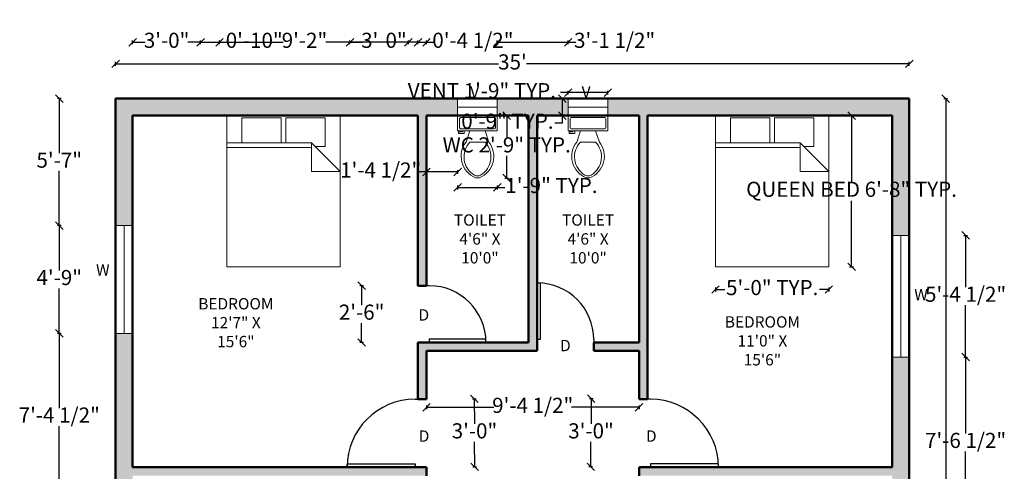
# Model space of a CAD drawing. Units: inches. Extents: x 2395 to 2921, y 528 to 1164.
# Tile 5 of 5: x 2395 to 2916, y 925 to 1164. Entities that reach past the tile are written whole.
import ezdxf

# ---------------------------------------------------------------- set-up
doc = ezdxf.new("R2010")
doc.units = ezdxf.units.IN
for name, color, linetype, lineweight in [('A-ANNO-DIMS', 2, 'Continuous', 18), ('A-ANNO-TEXT', 7, 'Continuous', 18), ('A-AREA-IDEN', 7, 'Continuous', 25), ('A-DOOR', 3, 'Continuous', 25), ('A-FLOR-FIXT', 9, 'Continuous', 18), ('A-FURN', 8, 'Continuous', 18), ('A-GLAZ', 4, 'Continuous', 18), ('A-WALL', 162, 'Continuous', 50), ('A-WALL-PATT', 162, 'Continuous', 13)]:
    doc.layers.add(name, color=color, linetype=linetype, lineweight=lineweight)
doc.styles.get("Standard").update_dxf_attribs({"font": 'arial.ttf'})
doc.dimstyles.new('ISO-25', dxfattribs={"dimtxt": 8, "dimasz": 4, "dimexe": 1, "dimexo": 1, "dimtad": 0, "dimtih": 1, "dimtoh": 1, "dimlunit": 3, "dimtxsty": 'Standard', "dimblk": 'OBLIQUE', "dimcen": 2.5, "dimadec": 0, "dimazin": 0, "dimtfac": 1, "dimtmove": 0, "dimatfit": 3, "dimfxl": 1, "dimfxlon": 1, "dimarcsym": 0})

# ---------------------------------------------------------------- blocks, each defined once
blk = doc.blocks.new('*U6')
for p, q in [((0, 0), (0, -6)), ((30, 0), (30, -6))]:
    blk.add_line(p, q)
blk.add_lwpolyline([(0, 0), (0, 30), (1.75, 30), (1.75, 0)], close=True)
blk.add_arc((0, 0), 30, 0, 90)
blk = doc.blocks.new('*U4')
for p, q in [((-30, 0), (-30, -6)), ((0, 0), (0, -6))]:
    blk.add_line(p, q)
blk.add_lwpolyline([(0, 0), (0, 30), (-1.75, 30), (-1.75, 0)], close=True)
blk.add_arc((0, 0), 30, 90, 180)
blk = doc.blocks.new('*U8')
for p, q in [((0, 0), (0, -6)), ((-36, 0), (-36, -6))]:
    blk.add_line(p, q)
blk.add_lwpolyline([(0, 0), (0, 36), (-1.75, 36), (-1.75, 0)], close=True)
blk.add_arc((0, 0), 36, 90, 180)
blk = doc.blocks.new('*U7')
for p, q in [((0, 0), (0, -6)), ((36, 0), (36, -6))]:
    blk.add_line(p, q)
blk.add_lwpolyline([(0, 0), (0, 36), (1.75, 36), (1.75, 0)], close=True)
blk.add_arc((0, 0), 36, 0, 90)
blk = doc.blocks.new('Toilet - top')
for p, q in [((9.5, -6), (9.5, -2)), ((-10, -8.5), (-8, -8.5)), ((-10, -9.5), (-10, -8.5)), ((-7, -9.5), (-10, -9.5)), ((-8, -8.5), (-8, -8)), ((-7, -8), (-7, -9.5)), ((-4, -8), (-6, -14)), ((4, -8), (6, -14)), ((4, -14), (-4, -14))]:
    blk.add_line(p, q)
blk.add_lwpolyline([(10.5, -8), (10.5, 0), (-10.5, 0), (-10.5, -8)], close=True)
for points in [[(-9.5, -2), (-9.5, -6)], [(8.5, -1), (-8.5, -1)], [(-8.5, -7), (8.5, -7)]]:
    blk.add_lwpolyline(points)
for centre, radius, start, end in [((-8.62, -1.88), 0.884, 81.8699, 188.1301), ((8.62, -1.88), 0.884, 351.8699, 98.1301), ((-8.62, -6.12), 0.884, 171.8699, 278.1301), ((8.62, -6.12), 0.884, 261.8699, 8.1301), ((3.52, -21.58), 12.17, 141.4691, 247.9714), ((4.2, -21.82), 11.33, 136.3677, 238.9468), ((-3.52, -21.58), 12.17, 292.0284, 38.5307), ((-4.2, -21.82), 11.33, 301.053, 43.6321), ((0, -27.88), 4, 245.7318, 294.2682), ((0, -29), 4, 254.8605, 285.1395)]:
    blk.add_arc(centre, radius, start, end)
blk = doc.blocks.new('Bed - Queen')
for p, q in [((0, -80.00003), (0, 0)), ((0, 0), (59.99999, 0)), ((59.99999, 0), (59.99999, -80.00003)), ((7.99999, -1.2), (28.79998, -1.2)), ((7.99999, -14.4), (7.99999, -1.2)), ((28.79998, -1.2), (28.79998, -14.4)), ((31.19999, -1.2), (51.99999, -1.2)), ((31.19999, -14.4), (31.19999, -1.2)), ((51.99999, -1.2), (51.99999, -16.4)), ((0, -14.4), (44.8, -14.4)), ((59.99999, -29.6), (44.8, -14.4)), ((44.8, -14.4), (44.8, -29.6)), ((44.8, -16.8), (0, -16.8)), ((51.99999, -16.4), (46.79936, -16.4)), ((44.8, -29.6), (59.99999, -29.6)), ((59.99999, -80.00003), (0, -80.00003))]:
    blk.add_line(p, q)
blk = doc.blocks.new('_Oblique')
at = {"color": 0, "linetype": 'ByBlock', "lineweight": -2}
blk.add_line((-0.5, -0.5), (0.5, 0.5), dxfattribs=at)
blk = doc.blocks.new('*D19')
at = {"layer": 'A-ANNO-DIMS', "color": 0, "lineweight": -2, "transparency": 16777216}
for p, q in [((2446.2, 1139.21), (2446.2, 1141.21)), ((2866.2, 1139.21), (2866.2, 1141.21)), ((2446.2, 1140.21), (2648.79, 1140.21)), ((2866.2, 1140.21), (2663.61, 1140.21))]:
    blk.add_line(p, q, dxfattribs=at)
at = {"layer": 'Defpoints', "color": 0, "transparency": 16777216}
for p in [(2866.2, 1140.21), (2446.2, 1121.85), (2866.2, 1121.85)]:
    blk.add_point(p, dxfattribs=at)
at = {"layer": 'A-ANNO-DIMS', "color": 0, "lineweight": -2, "transparency": 16777216, "xscale": 4, "yscale": 4, "zscale": 4, "rotation": 180}
blk.add_blockref('_Oblique', (2446.2, 1140.21), dxfattribs=at)
at = {"layer": 'A-ANNO-DIMS', "color": 0, "lineweight": -2, "transparency": 16777216, "xscale": 4, "yscale": 4, "zscale": 4}
blk.add_blockref('_Oblique', (2866.2, 1140.21), dxfattribs=at)
at = {"layer": 'A-ANNO-DIMS', "color": 0, "transparency": 16777216, "insert": (2656.2, 1140.21), "char_height": 8, "attachment_point": 5}
blk.add_mtext("35'", dxfattribs=at)
blk = doc.blocks.new('*D20')
at = {"layer": 'A-ANNO-DIMS', "color": 0, "lineweight": -2, "transparency": 16777216}
for p, q in [((2884.49, 1121.85), (2886.49, 1121.85)), ((2885.49, 1121.85), (2885.49, 850.56)), ((2885.49, 569.85), (2885.49, 841.14)), ((2884.49, 569.85), (2886.49, 569.85))]:
    blk.add_line(p, q, dxfattribs=at)
at = {"layer": 'Defpoints', "color": 0, "transparency": 16777216}
for p in [(2866.2, 1121.85), (2866.2, 569.85), (2885.49, 569.85)]:
    blk.add_point(p, dxfattribs=at)
at = {"layer": 'A-ANNO-DIMS', "color": 0, "lineweight": -2, "transparency": 16777216, "xscale": 4, "yscale": 4, "zscale": 4}
for p, rotation in [((2885.49, 1121.85), 90), ((2885.49, 569.85), 270)]:
    blk.add_blockref('_Oblique', p, dxfattribs=dict(at, rotation=rotation))
at = {"layer": 'A-ANNO-DIMS', "color": 0, "transparency": 16777216, "insert": (2885.49, 845.85), "char_height": 8, "attachment_point": 5}
blk.add_mtext("46'", dxfattribs=at)
blk = doc.blocks.new('VENT-WINDOW-21IN')
for p, q in [((0, 0), (0, 9)), ((21, 0), (21, 9)), ((0, 4.5), (21, 4.5))]:
    blk.add_line(p, q)
blk = doc.blocks.new('*D22')
at = {"layer": 'A-ANNO-DIMS', "color": 0, "lineweight": -2, "transparency": 16777216}
for p, q in [((2834.65, 1112.85), (2836.65, 1112.85)), ((2835.65, 1112.85), (2835.65, 1077.86)), ((2835.65, 1032.85), (2835.65, 1067.85)), ((2834.65, 1032.85), (2836.65, 1032.85))]:
    blk.add_line(p, q, dxfattribs=at)
at = {"layer": 'Defpoints', "color": 0, "transparency": 16777216}
for p in [(2823.65, 1112.85), (2835.65, 1112.85), (2823.65, 1032.85)]:
    blk.add_point(p, dxfattribs=at)
at = {"layer": 'A-ANNO-DIMS', "color": 0, "lineweight": -2, "transparency": 16777216, "xscale": 4, "yscale": 4, "zscale": 4}
for p, rotation in [((2835.65, 1112.85), 90), ((2835.65, 1032.85), 270)]:
    blk.add_blockref('_Oblique', p, dxfattribs=dict(at, rotation=rotation))
at = {"layer": 'A-ANNO-DIMS', "color": 0, "transparency": 16777216, "insert": (2835.65, 1072.85), "char_height": 8, "attachment_point": 5}
blk.add_mtext('QUEEN BED 6\'-8" TYP.', dxfattribs=at)
blk = doc.blocks.new('*D23')
at = {"layer": 'A-ANNO-DIMS', "color": 0, "lineweight": -2, "transparency": 16777216}
for p, q in [((2763.65, 1021.85), (2763.65, 1019.85)), ((2823.65, 1021.85), (2823.65, 1019.85)), ((2763.65, 1020.85), (2768.64, 1020.85)), ((2823.65, 1020.85), (2818.66, 1020.85))]:
    blk.add_line(p, q, dxfattribs=at)
at = {"layer": 'Defpoints', "color": 0, "transparency": 16777216}
for p in [(2763.65, 1032.85), (2823.65, 1032.85), (2823.65, 1020.85)]:
    blk.add_point(p, dxfattribs=at)
at = {"layer": 'A-ANNO-DIMS', "color": 0, "lineweight": -2, "transparency": 16777216, "xscale": 4, "yscale": 4, "zscale": 4, "rotation": 180}
blk.add_blockref('_Oblique', (2763.65, 1020.85), dxfattribs=at)
at = {"layer": 'A-ANNO-DIMS', "color": 0, "lineweight": -2, "transparency": 16777216, "xscale": 4, "yscale": 4, "zscale": 4}
blk.add_blockref('_Oblique', (2823.65, 1020.85), dxfattribs=at)
at = {"layer": 'A-ANNO-DIMS', "color": 0, "transparency": 16777216, "insert": (2793.65, 1020.85), "char_height": 8, "attachment_point": 5}
blk.add_mtext('5\'-0" TYP.', dxfattribs=at)
blk = doc.blocks.new('*D24')
at = {"layer": 'A-ANNO-DIMS', "color": 0, "lineweight": -2, "transparency": 16777216}
for p, q in [((2652.16, 1112.85), (2654.16, 1112.85)), ((2653.16, 1112.85), (2653.16, 1101.09)), ((2653.16, 1079.81), (2653.16, 1091.57)), ((2652.16, 1079.81), (2654.16, 1079.81))]:
    blk.add_line(p, q, dxfattribs=at)
at = {"layer": 'Defpoints', "color": 0, "transparency": 16777216}
for p in [(2648.2, 1112.85), (2653.16, 1112.85), (2648.2, 1079.81)]:
    blk.add_point(p, dxfattribs=at)
at = {"layer": 'A-ANNO-DIMS', "color": 0, "lineweight": -2, "transparency": 16777216, "xscale": 4, "yscale": 4, "zscale": 4}
for p, rotation in [((2653.16, 1112.85), 90), ((2653.16, 1079.81), 270)]:
    blk.add_blockref('_Oblique', p, dxfattribs=dict(at, rotation=rotation))
at = {"layer": 'A-ANNO-DIMS', "color": 0, "transparency": 16777216, "insert": (2653.16, 1096.33), "char_height": 8, "attachment_point": 5}
blk.add_mtext('WC 2\'-9" TYP.', dxfattribs=at)
blk = doc.blocks.new('*D25')
at = {"layer": 'A-ANNO-DIMS', "color": 0, "lineweight": -2, "transparency": 16777216}
for p, q in [((2627.2, 1075.85), (2627.2, 1073.85)), ((2627.2, 1074.85), (2648.2, 1074.85)), ((2648.2, 1075.85), (2648.2, 1073.85)), ((2648.2, 1074.85), (2652.2, 1074.85))]:
    blk.add_line(p, q, dxfattribs=at)
at = {"layer": 'Defpoints', "color": 0, "transparency": 16777216}
for p in [(2627.2, 1079.81), (2648.2, 1079.81), (2648.2, 1074.85)]:
    blk.add_point(p, dxfattribs=at)
at = {"layer": 'A-ANNO-DIMS', "color": 0, "lineweight": -2, "transparency": 16777216, "xscale": 4, "yscale": 4, "zscale": 4, "rotation": 180}
blk.add_blockref('_Oblique', (2627.2, 1074.85), dxfattribs=at)
at = {"layer": 'A-ANNO-DIMS', "color": 0, "lineweight": -2, "transparency": 16777216, "xscale": 4, "yscale": 4, "zscale": 4}
blk.add_blockref('_Oblique', (2648.2, 1074.85), dxfattribs=at)
at = {"layer": 'A-ANNO-DIMS', "color": 0, "transparency": 16777216, "insert": (2676.83, 1074.85), "char_height": 8, "attachment_point": 5}
blk.add_mtext('1\'-9" TYP.', dxfattribs=at)
blk = doc.blocks.new('*D26')
at = {"layer": 'A-ANNO-DIMS', "color": 0, "lineweight": -2, "transparency": 16777216}
for p, q in [((2685.7, 1124), (2685.7, 1126)), ((2706.7, 1124), (2706.7, 1126)), ((2685.7, 1125), (2681.7, 1125)), ((2706.7, 1125), (2685.7, 1125))]:
    blk.add_line(p, q, dxfattribs=at)
at = {"layer": 'Defpoints', "color": 0, "transparency": 16777216}
for p in [(2685.7, 1125), (2685.7, 1121.85), (2706.7, 1121.85)]:
    blk.add_point(p, dxfattribs=at)
at = {"layer": 'A-ANNO-DIMS', "color": 0, "lineweight": -2, "transparency": 16777216, "xscale": 4, "yscale": 4, "zscale": 4, "rotation": 180}
blk.add_blockref('_Oblique', (2685.7, 1125), dxfattribs=at)
at = {"layer": 'A-ANNO-DIMS', "color": 0, "lineweight": -2, "transparency": 16777216, "xscale": 4, "yscale": 4, "zscale": 4}
blk.add_blockref('_Oblique', (2706.7, 1125), dxfattribs=at)
at = {"layer": 'A-ANNO-DIMS', "color": 0, "transparency": 16777216, "insert": (2640.03, 1125), "char_height": 8, "attachment_point": 5}
blk.add_mtext('VENT 1\'-9" TYP.', dxfattribs=at)
blk = doc.blocks.new('*D27')
at = {"layer": 'A-ANNO-DIMS', "color": 0, "lineweight": -2, "transparency": 16777216}
for p, q in [((2683.55, 1121.85), (2681.55, 1121.85)), ((2682.55, 1121.85), (2682.55, 1112.85)), ((2683.55, 1112.85), (2681.55, 1112.85)), ((2682.55, 1112.85), (2682.55, 1108.85)), ((2682.55, 1108.85), (2678.55, 1108.85))]:
    blk.add_line(p, q, dxfattribs=at)
at = {"layer": 'Defpoints', "color": 0, "transparency": 16777216}
for p in [(2685.7, 1121.85), (2682.55, 1112.85), (2685.7, 1112.85)]:
    blk.add_point(p, dxfattribs=at)
at = {"layer": 'A-ANNO-DIMS', "color": 0, "lineweight": -2, "transparency": 16777216, "xscale": 4, "yscale": 4, "zscale": 4}
for p, rotation in [((2682.55, 1121.85), 90), ((2682.55, 1112.85), 270)]:
    blk.add_blockref('_Oblique', p, dxfattribs=dict(at, rotation=rotation))
at = {"layer": 'A-ANNO-DIMS', "color": 0, "transparency": 16777216, "insert": (2653.54, 1108.85), "char_height": 8, "attachment_point": 5}
blk.add_mtext('0\'-9" TYP.', dxfattribs=at)
blk = doc.blocks.new('*D51')
at = {"layer": 'A-ANNO-DIMS', "color": 0, "lineweight": -2, "transparency": 16777216}
for p, q in [((2606.2, 1150.65), (2606.2, 1152.65)), ((2606.2, 1151.65), (2610.7, 1151.65)), ((2610.7, 1150.65), (2610.7, 1152.65)), ((2610.7, 1151.65), (2614.7, 1151.65))]:
    blk.add_line(p, q, dxfattribs=at)
at = {"layer": 'Defpoints', "color": 0, "transparency": 16777216}
for p in [(2610.7, 1151.65), (2606.2, 578.85), (2610.7, 578.85)]:
    blk.add_point(p, dxfattribs=at)
at = {"layer": 'A-ANNO-DIMS', "color": 0, "lineweight": -2, "transparency": 16777216, "xscale": 4, "yscale": 4, "zscale": 4, "rotation": 180}
blk.add_blockref('_Oblique', (2606.2, 1151.65), dxfattribs=at)
at = {"layer": 'A-ANNO-DIMS', "color": 0, "lineweight": -2, "transparency": 16777216, "xscale": 4, "yscale": 4, "zscale": 4}
blk.add_blockref('_Oblique', (2610.7, 1151.65), dxfattribs=at)
at = {"layer": 'A-ANNO-DIMS', "color": 0, "transparency": 16777216, "insert": (2635.28, 1151.65), "char_height": 8, "attachment_point": 5}
blk.add_mtext('0\'-4 1/2"', dxfattribs=at)
blk = doc.blocks.new('*D53')
at = {"layer": 'A-ANNO-DIMS', "color": 0, "lineweight": -2, "transparency": 16777216}
for p, q in [((2455.2, 1150.65), (2455.2, 1152.65)), ((2455.2, 1151.65), (2461.94, 1151.65)), ((2491.2, 1151.65), (2484.46, 1151.65)), ((2491.2, 1150.65), (2491.2, 1152.65))]:
    blk.add_line(p, q, dxfattribs=at)
at = {"layer": 'Defpoints', "color": 0, "transparency": 16777216}
for p in [(2491.2, 1151.65), (2455.2, 922.35), (2491.2, 922.35)]:
    blk.add_point(p, dxfattribs=at)
at = {"layer": 'A-ANNO-DIMS', "color": 0, "lineweight": -2, "transparency": 16777216, "xscale": 4, "yscale": 4, "zscale": 4, "rotation": 180}
blk.add_blockref('_Oblique', (2455.2, 1151.65), dxfattribs=at)
at = {"layer": 'A-ANNO-DIMS', "color": 0, "lineweight": -2, "transparency": 16777216, "xscale": 4, "yscale": 4, "zscale": 4}
blk.add_blockref('_Oblique', (2491.2, 1151.65), dxfattribs=at)
at = {"layer": 'A-ANNO-DIMS', "color": 0, "transparency": 16777216, "insert": (2473.2, 1151.65), "char_height": 8, "attachment_point": 5}
blk.add_mtext('3\'-0"', dxfattribs=at)
blk = doc.blocks.new('*D54')
at = {"layer": 'A-ANNO-DIMS', "color": 0, "lineweight": -2, "transparency": 16777216}
for p, q in [((2491.2, 1150.65), (2491.2, 1152.65)), ((2491.2, 1151.65), (2534.91, 1151.65)), ((2601.13, 1151.65), (2557.42, 1151.65)), ((2601.13, 1150.65), (2601.13, 1152.65))]:
    blk.add_line(p, q, dxfattribs=at)
at = {"layer": 'Defpoints', "color": 0, "transparency": 16777216}
for p in [(2601.13, 1151.65), (2491.2, 922.35), (2601.13, 922.35)]:
    blk.add_point(p, dxfattribs=at)
at = {"layer": 'A-ANNO-DIMS', "color": 0, "lineweight": -2, "transparency": 16777216, "xscale": 4, "yscale": 4, "zscale": 4, "rotation": 180}
blk.add_blockref('_Oblique', (2491.2, 1151.65), dxfattribs=at)
at = {"layer": 'A-ANNO-DIMS', "color": 0, "lineweight": -2, "transparency": 16777216, "xscale": 4, "yscale": 4, "zscale": 4}
blk.add_blockref('_Oblique', (2601.13, 1151.65), dxfattribs=at)
at = {"layer": 'A-ANNO-DIMS', "color": 0, "transparency": 16777216, "insert": (2546.16, 1151.65), "char_height": 8, "attachment_point": 5}
blk.add_mtext('9\'-2"', dxfattribs=at)
blk = doc.blocks.new('*D55')
at = {"layer": 'A-ANNO-DIMS', "color": 0, "lineweight": -2, "transparency": 16777216}
for p, q in [((2491.2, 1150.65), (2491.2, 1152.65)), ((2491.2, 1151.65), (2501.19, 1151.65)), ((2501.19, 1150.65), (2501.19, 1152.65)), ((2501.19, 1151.65), (2505.19, 1151.65))]:
    blk.add_line(p, q, dxfattribs=at)
at = {"layer": 'Defpoints', "color": 0, "transparency": 16777216}
for p in [(2501.19, 1151.65), (2491.2, 842.85), (2501.19, 842.85)]:
    blk.add_point(p, dxfattribs=at)
at = {"layer": 'A-ANNO-DIMS', "color": 0, "lineweight": -2, "transparency": 16777216, "xscale": 4, "yscale": 4, "zscale": 4, "rotation": 180}
blk.add_blockref('_Oblique', (2491.2, 1151.65), dxfattribs=at)
at = {"layer": 'A-ANNO-DIMS', "color": 0, "lineweight": -2, "transparency": 16777216, "xscale": 4, "yscale": 4, "zscale": 4}
blk.add_blockref('_Oblique', (2501.19, 1151.65), dxfattribs=at)
at = {"layer": 'A-ANNO-DIMS', "color": 0, "transparency": 16777216, "insert": (2519.56, 1151.65), "char_height": 8, "attachment_point": 5}
blk.add_mtext('0\'-10"', dxfattribs=at)
blk = doc.blocks.new('*D56')
at = {"layer": 'A-ANNO-DIMS', "color": 0, "lineweight": -2, "transparency": 16777216}
for p, q in [((2417.4, 1121.85), (2415.4, 1121.85)), ((2416.4, 1121.85), (2416.4, 1092.94)), ((2416.4, 1054.65), (2416.4, 1083.56)), ((2417.4, 1054.65), (2415.4, 1054.65))]:
    blk.add_line(p, q, dxfattribs=at)
at = {"layer": 'Defpoints', "color": 0, "transparency": 16777216}
for p in [(2446.2, 1121.85), (2416.4, 1054.65), (2446.2, 1054.65)]:
    blk.add_point(p, dxfattribs=at)
at = {"layer": 'A-ANNO-DIMS', "color": 0, "lineweight": -2, "transparency": 16777216, "xscale": 4, "yscale": 4, "zscale": 4}
for p, rotation in [((2416.4, 1121.85), 90), ((2416.4, 1054.65), 270)]:
    blk.add_blockref('_Oblique', p, dxfattribs=dict(at, rotation=rotation))
at = {"layer": 'A-ANNO-DIMS', "color": 0, "transparency": 16777216, "insert": (2416.4, 1088.25), "char_height": 8, "attachment_point": 5}
blk.add_mtext('5\'-7"', dxfattribs=at)
blk = doc.blocks.new('*D57')
at = {"layer": 'A-ANNO-DIMS', "color": 0, "lineweight": -2, "transparency": 16777216}
for p, q in [((2417.4, 1054.65), (2415.4, 1054.65)), ((2416.4, 1054.65), (2416.4, 1030.86)), ((2416.4, 997.65), (2416.4, 1021.44)), ((2417.4, 997.65), (2415.4, 997.65))]:
    blk.add_line(p, q, dxfattribs=at)
at = {"layer": 'Defpoints', "color": 0, "transparency": 16777216}
for p in [(2446.2, 1054.65), (2416.4, 997.65), (2446.2, 997.65)]:
    blk.add_point(p, dxfattribs=at)
at = {"layer": 'A-ANNO-DIMS', "color": 0, "lineweight": -2, "transparency": 16777216, "xscale": 4, "yscale": 4, "zscale": 4}
for p, rotation in [((2416.4, 1054.65), 90), ((2416.4, 997.65), 270)]:
    blk.add_blockref('_Oblique', p, dxfattribs=dict(at, rotation=rotation))
at = {"layer": 'A-ANNO-DIMS', "color": 0, "transparency": 16777216, "insert": (2416.4, 1026.15), "char_height": 8, "attachment_point": 5}
blk.add_mtext('4\'-9"', dxfattribs=at)
blk = doc.blocks.new('*D58')
at = {"layer": 'A-ANNO-DIMS', "color": 0, "lineweight": -2, "transparency": 16777216}
for p, q in [((2417.4, 997.65), (2415.4, 997.65)), ((2416.4, 997.65), (2416.4, 958.18)), ((2416.4, 909.18), (2416.4, 948.66)), ((2417.4, 909.18), (2415.4, 909.18))]:
    blk.add_line(p, q, dxfattribs=at)
at = {"layer": 'Defpoints', "color": 0, "transparency": 16777216}
for p in [(2446.2, 997.65), (2416.4, 909.18), (2446.2, 909.18)]:
    blk.add_point(p, dxfattribs=at)
at = {"layer": 'A-ANNO-DIMS', "color": 0, "lineweight": -2, "transparency": 16777216, "xscale": 4, "yscale": 4, "zscale": 4}
for p, rotation in [((2416.4, 997.65), 90), ((2416.4, 909.18), 270)]:
    blk.add_blockref('_Oblique', p, dxfattribs=dict(at, rotation=rotation))
at = {"layer": 'A-ANNO-DIMS', "color": 0, "transparency": 16777216, "insert": (2416.4, 953.42), "char_height": 8, "attachment_point": 5}
blk.add_mtext('7\'-4 1/2"', dxfattribs=at)
blk = doc.blocks.new('*D68')
at = {"layer": 'A-ANNO-DIMS', "color": 0, "lineweight": -2, "transparency": 16777216}
for p, q in [((2895, 985.13), (2897, 985.13)), ((2896, 985.13), (2896, 944.76)), ((2896, 894.87), (2896, 935.24)), ((2895, 894.87), (2897, 894.87))]:
    blk.add_line(p, q, dxfattribs=at)
at = {"layer": 'Defpoints', "color": 0, "transparency": 16777216}
for p in [(2866.2, 985.13), (2896, 985.13), (2866.2, 894.87)]:
    blk.add_point(p, dxfattribs=at)
at = {"layer": 'A-ANNO-DIMS', "color": 0, "lineweight": -2, "transparency": 16777216, "xscale": 4, "yscale": 4, "zscale": 4}
for p, rotation in [((2896, 985.13), 90), ((2896, 894.87), 270)]:
    blk.add_blockref('_Oblique', p, dxfattribs=dict(at, rotation=rotation))
at = {"layer": 'A-ANNO-DIMS', "color": 0, "transparency": 16777216, "insert": (2896, 940), "char_height": 8, "attachment_point": 5}
blk.add_mtext('7\'-6 1/2"', dxfattribs=at)
blk = doc.blocks.new('*D69')
at = {"layer": 'A-ANNO-DIMS', "color": 0, "lineweight": -2, "transparency": 16777216}
for p, q in [((2895, 1049.51), (2897, 1049.51)), ((2896, 1049.51), (2896, 1022.08)), ((2896, 985.13), (2896, 1012.56)), ((2895, 985.13), (2897, 985.13))]:
    blk.add_line(p, q, dxfattribs=at)
at = {"layer": 'Defpoints', "color": 0, "transparency": 16777216}
for p in [(2866.2, 1049.51), (2896, 1049.51), (2866.2, 985.13)]:
    blk.add_point(p, dxfattribs=at)
at = {"layer": 'A-ANNO-DIMS', "color": 0, "lineweight": -2, "transparency": 16777216, "xscale": 4, "yscale": 4, "zscale": 4}
for p, rotation in [((2896, 1049.51), 90), ((2896, 985.13), 270)]:
    blk.add_blockref('_Oblique', p, dxfattribs=dict(at, rotation=rotation))
at = {"layer": 'A-ANNO-DIMS', "color": 0, "transparency": 16777216, "insert": (2896, 1017.32), "char_height": 8, "attachment_point": 5}
blk.add_mtext('5\'-4 1/2"', dxfattribs=at)
blk = doc.blocks.new('*D70')
at = {"layer": 'A-ANNO-DIMS', "color": 0, "lineweight": -2, "transparency": 16777216}
for p, q in [((2610.7, 1084.05), (2610.7, 1082.05)), ((2627.2, 1084.05), (2627.2, 1082.05)), ((2610.7, 1083.05), (2606.7, 1083.05)), ((2627.2, 1083.05), (2610.7, 1083.05))]:
    blk.add_line(p, q, dxfattribs=at)
at = {"layer": 'Defpoints', "color": 0, "transparency": 16777216}
for p in [(2610.7, 1112.85), (2627.2, 1112.85), (2610.7, 1083.05)]:
    blk.add_point(p, dxfattribs=at)
at = {"layer": 'A-ANNO-DIMS', "color": 0, "lineweight": -2, "transparency": 16777216, "xscale": 4, "yscale": 4, "zscale": 4, "rotation": 180}
blk.add_blockref('_Oblique', (2610.7, 1083.05), dxfattribs=at)
at = {"layer": 'A-ANNO-DIMS', "color": 0, "lineweight": -2, "transparency": 16777216, "xscale": 4, "yscale": 4, "zscale": 4}
blk.add_blockref('_Oblique', (2627.2, 1083.05), dxfattribs=at)
at = {"layer": 'A-ANNO-DIMS', "color": 0, "transparency": 16777216, "insert": (2586.5, 1083.05), "char_height": 8, "attachment_point": 5}
blk.add_mtext('1\'-4 1/2"', dxfattribs=at)
blk = doc.blocks.new('*D71')
at = {"layer": 'A-ANNO-DIMS', "color": 0, "lineweight": -2, "transparency": 16777216}
for p, q in [((2648.2, 1150.65), (2648.2, 1152.65)), ((2648.2, 1151.65), (2685.7, 1151.65)), ((2685.7, 1150.65), (2685.7, 1152.65)), ((2685.7, 1151.65), (2689.7, 1151.65))]:
    blk.add_line(p, q, dxfattribs=at)
at = {"layer": 'Defpoints', "color": 0, "transparency": 16777216}
for p in [(2685.7, 1151.65), (2648.2, 1121.85), (2685.7, 1121.85)]:
    blk.add_point(p, dxfattribs=at)
at = {"layer": 'A-ANNO-DIMS', "color": 0, "lineweight": -2, "transparency": 16777216, "xscale": 4, "yscale": 4, "zscale": 4, "rotation": 180}
blk.add_blockref('_Oblique', (2648.2, 1151.65), dxfattribs=at)
at = {"layer": 'A-ANNO-DIMS', "color": 0, "lineweight": -2, "transparency": 16777216, "xscale": 4, "yscale": 4, "zscale": 4}
blk.add_blockref('_Oblique', (2685.7, 1151.65), dxfattribs=at)
at = {"layer": 'A-ANNO-DIMS', "color": 0, "transparency": 16777216, "insert": (2710.28, 1151.65), "char_height": 8, "attachment_point": 5}
blk.add_mtext('3\'-1 1/2"', dxfattribs=at)
blk = doc.blocks.new('*D72')
at = {"layer": 'A-ANNO-DIMS', "color": 0, "lineweight": -2, "transparency": 16777216}
for p, q in [((2577.4, 1022.85), (2575.4, 1022.85)), ((2576.4, 1022.85), (2576.4, 1012.56)), ((2576.4, 992.85), (2576.4, 1003.14)), ((2577.4, 992.85), (2575.4, 992.85))]:
    blk.add_line(p, q, dxfattribs=at)
at = {"layer": 'Defpoints', "color": 0, "transparency": 16777216}
for p in [(2576.4, 1022.85), (2606.2, 1022.85), (2606.2, 992.85)]:
    blk.add_point(p, dxfattribs=at)
at = {"layer": 'A-ANNO-DIMS', "color": 0, "lineweight": -2, "transparency": 16777216, "xscale": 4, "yscale": 4, "zscale": 4}
for p, rotation in [((2576.4, 1022.85), 90), ((2576.4, 992.85), 270)]:
    blk.add_blockref('_Oblique', p, dxfattribs=dict(at, rotation=rotation))
at = {"layer": 'A-ANNO-DIMS', "color": 0, "transparency": 16777216, "insert": (2576.4, 1007.85), "char_height": 8, "attachment_point": 5}
blk.add_mtext('2\'-6"', dxfattribs=at)
blk = doc.blocks.new('*D73')
at = {"layer": 'A-ANNO-DIMS', "color": 0, "lineweight": -2, "transparency": 16777216}
for p, q in [((2669.2, 541.05), (2669.2, 539.05)), ((2669.2, 540.05), (2672.87, 540.05)), ((2699.2, 540.05), (2695.53, 540.05)), ((2699.2, 541.05), (2699.2, 539.05))]:
    blk.add_line(p, q, dxfattribs=at)
at = {"layer": 'Defpoints', "color": 0, "transparency": 16777216}
for p in [(2669.2, 988.35), (2699.2, 988.35), (2699.2, 540.05)]:
    blk.add_point(p, dxfattribs=at)
at = {"layer": 'A-ANNO-DIMS', "color": 0, "lineweight": -2, "transparency": 16777216, "xscale": 4, "yscale": 4, "zscale": 4, "rotation": 180}
blk.add_blockref('_Oblique', (2669.2, 540.05), dxfattribs=at)
at = {"layer": 'A-ANNO-DIMS', "color": 0, "lineweight": -2, "transparency": 16777216, "xscale": 4, "yscale": 4, "zscale": 4}
blk.add_blockref('_Oblique', (2699.2, 540.05), dxfattribs=at)
at = {"layer": 'A-ANNO-DIMS', "color": 0, "transparency": 16777216, "insert": (2684.2, 540.05), "char_height": 8, "attachment_point": 5}
blk.add_mtext('2\'-6"', dxfattribs=at)
blk = doc.blocks.new('*D74')
at = {"layer": 'A-ANNO-DIMS', "color": 0, "lineweight": -2, "transparency": 16777216}
for p, q in [((2635, 963.05), (2637, 963.07)), ((2636, 963.06), (2636.09, 949.77)), ((2636.25, 927.06), (2636.16, 940.35)), ((2635.25, 927.05), (2637.25, 927.07))]:
    blk.add_line(p, q, dxfattribs=at)
at = {"layer": 'Defpoints', "color": 0, "transparency": 16777216}
for p in [(2606.2, 962.85), (2606.45, 926.85), (2636.25, 927.06)]:
    blk.add_point(p, dxfattribs=at)
at = {"layer": 'A-ANNO-DIMS', "color": 0, "lineweight": -2, "transparency": 16777216, "xscale": 4, "yscale": 4, "zscale": 4}
for p, rotation in [((2636, 963.06), 90.39788096183455), ((2636.25, 927.06), 270.3978809618346)]:
    blk.add_blockref('_Oblique', p, dxfattribs=dict(at, rotation=rotation))
at = {"layer": 'A-ANNO-DIMS', "color": 0, "transparency": 16777216, "insert": (2636.12, 945.06), "char_height": 8, "attachment_point": 5}
blk.add_mtext('3\'-0"', dxfattribs=at)
blk = doc.blocks.new('*D75')
at = {"layer": 'A-ANNO-DIMS', "color": 0, "lineweight": -2, "transparency": 16777216}
for p, q in [((2698.9, 963.05), (2696.9, 963.07)), ((2697.9, 963.06), (2697.81, 949.77)), ((2697.65, 927.06), (2697.74, 940.35)), ((2698.65, 927.05), (2696.65, 927.07))]:
    blk.add_line(p, q, dxfattribs=at)
at = {"layer": 'Defpoints', "color": 0, "transparency": 16777216}
for p in [(2697.9, 963.06), (2727.7, 962.85), (2727.45, 926.85)]:
    blk.add_point(p, dxfattribs=at)
at = {"layer": 'A-ANNO-DIMS', "color": 0, "lineweight": -2, "transparency": 16777216, "xscale": 4, "yscale": 4, "zscale": 4}
for p, rotation in [((2697.9, 963.06), 89.6021190381654), ((2697.65, 927.06), 269.6021190381654)]:
    blk.add_blockref('_Oblique', p, dxfattribs=dict(at, rotation=rotation))
at = {"layer": 'A-ANNO-DIMS', "color": 0, "transparency": 16777216, "insert": (2697.78, 945.06), "char_height": 8, "attachment_point": 5}
blk.add_mtext('3\'-0"', dxfattribs=at)
blk = doc.blocks.new('*D78')
at = {"layer": 'A-ANNO-DIMS', "color": 0, "lineweight": -2, "transparency": 16777216}
for p, q in [((2570.2, 1150.65), (2570.2, 1152.65)), ((2570.2, 1151.65), (2576.94, 1151.65)), ((2606.2, 1151.65), (2599.46, 1151.65)), ((2606.2, 1150.65), (2606.2, 1152.65))]:
    blk.add_line(p, q, dxfattribs=at)
at = {"layer": 'Defpoints', "color": 0, "transparency": 16777216}
for p in [(2606.2, 1151.65), (2570.2, 734.85), (2606.2, 735.1)]:
    blk.add_point(p, dxfattribs=at)
at = {"layer": 'A-ANNO-DIMS', "color": 0, "lineweight": -2, "transparency": 16777216, "xscale": 4, "yscale": 4, "zscale": 4, "rotation": 180}
blk.add_blockref('_Oblique', (2570.2, 1151.65), dxfattribs=at)
at = {"layer": 'A-ANNO-DIMS', "color": 0, "lineweight": -2, "transparency": 16777216, "xscale": 4, "yscale": 4, "zscale": 4}
blk.add_blockref('_Oblique', (2606.2, 1151.65), dxfattribs=at)
at = {"layer": 'A-ANNO-DIMS', "color": 0, "transparency": 16777216, "insert": (2588.2, 1151.65), "char_height": 8, "attachment_point": 5}
blk.add_mtext('3\'-0"', dxfattribs=at)
blk = doc.blocks.new('*D79')
at = {"layer": 'A-ANNO-DIMS', "color": 0, "lineweight": -2, "transparency": 16777216}
for p, q in [((2610.7, 959.55), (2610.7, 957.55)), ((2723.2, 959.55), (2723.2, 957.55)), ((2610.7, 958.55), (2646.37, 958.55)), ((2723.2, 958.55), (2687.53, 958.55))]:
    blk.add_line(p, q, dxfattribs=at)
at = {"layer": 'Defpoints', "color": 0, "transparency": 16777216}
for p in [(2610.7, 988.35), (2723.2, 988.35), (2610.7, 958.55)]:
    blk.add_point(p, dxfattribs=at)
at = {"layer": 'A-ANNO-DIMS', "color": 0, "lineweight": -2, "transparency": 16777216, "xscale": 4, "yscale": 4, "zscale": 4, "rotation": 180}
blk.add_blockref('_Oblique', (2610.7, 958.55), dxfattribs=at)
at = {"layer": 'A-ANNO-DIMS', "color": 0, "lineweight": -2, "transparency": 16777216, "xscale": 4, "yscale": 4, "zscale": 4}
blk.add_blockref('_Oblique', (2723.2, 958.55), dxfattribs=at)
at = {"layer": 'A-ANNO-DIMS', "color": 0, "transparency": 16777216, "insert": (2666.95, 958.55), "char_height": 8, "attachment_point": 5}
blk.add_mtext('9\'-4 1/2"', dxfattribs=at)

msp = doc.modelspace()

# ---------------------------------------------------------------- hatches: boundary and pattern name
at = {"layer": 'A-WALL-PATT'}
h = msp.add_hatch(color=256, dxfattribs=at)
h.dxf.hatch_style = 1
h.paths.add_polyline_path([(2627.2, 1121.853), (2446.2, 1121.853), (2446.2, 1054.648), (2455.2, 1054.648), (2455.2, 1112.853), (2606.2, 1112.853), (2606.2, 1022.853), (2610.7, 1022.853), (2610.7, 1112.853), (2627.2, 1112.853)])
h.paths.add_polyline_path([(2685.7, 1121.853), (2648.2, 1121.853), (2648.2, 1112.853), (2664.7, 1112.853), (2664.7, 992.853), (2606.2, 992.853), (2606.2, 962.853), (2610.7, 962.853), (2610.7, 988.353), (2669.2, 988.353), (2669.2, 994.353), (2669.2, 1024.353), (2669.2, 1112.853), (2685.7, 1112.853)])
h.paths.add_polyline_path([(2866.2, 1121.853), (2706.7, 1121.853), (2706.7, 1112.853), (2723.2, 1112.853), (2723.2, 992.853), (2699.2, 992.853), (2699.2, 988.353), (2723.2, 988.353), (2723.2, 962.853), (2727.7, 962.853), (2727.7, 1112.853), (2857.2, 1112.853), (2857.2, 1049.508), (2866.2, 1049.508)])
h.paths.add_polyline_path([(2866.2, 985.129), (2857.2, 985.129), (2857.2, 926.853), (2723.2, 926.853), (2723.2, 922.353), (2729.2, 922.353), (2765.2, 922.353), (2857.2, 922.353), (2857.2, 894.873), (2866.2, 894.873)])
h.paths.add_polyline_path([(2455.2, 997.652), (2446.2, 997.652), (2446.2, 909.181), (2455.2, 908.938), (2455.2, 922.353), (2610.7, 922.353), (2610.7, 926.853), (2455.2, 926.853)])
h.paths.add_polyline_path([(2455.2, 838.353), (2610.7, 838.353), (2610.7, 842.853), (2455.2, 842.853), (2455.2, 856.236), (2446.2, 856.236), (2446.2, 815.427), (2455.2, 815.427)])
h.paths.add_polyline_path([(2455.2, 772.706), (2446.2, 772.706), (2446.2, 569.853), (2505.031, 569.853), (2505.031, 578.853), (2455.2, 578.853), (2455.2, 734.853), (2570.2, 734.853), (2570.2, 739.353), (2568.7, 739.353), (2568.7, 806.353), (2564.2, 806.353), (2564.2, 739.353), (2455.2, 739.353)])
h.paths.add_polyline_path([(2656.2, 578.853), (2610.7, 578.853), (2610.7, 739.353), (2606.2, 739.353), (2606.2, 578.853), (2565.031, 578.853), (2565.031, 569.853), (2656.2, 569.853)])
h.paths.add_polyline_path([(2733.198, 578.853), (2716.2, 578.853), (2716.2, 569.853), (2733.198, 569.853)])
h.paths.add_polyline_path([(2801.188, 578.853), (2764.893, 578.853), (2764.893, 569.853), (2801.188, 569.853)])
h.paths.add_polyline_path([(2866.2, 616.306), (2857.2, 616.306), (2857.2, 578.853), (2836.314, 578.853), (2836.314, 569.853), (2866.2, 569.853)])
h.paths.add_polyline_path([(2866.2, 727.906), (2857.2, 727.906), (2857.2, 670.095), (2866.2, 670.095)])
h.paths.add_polyline_path([(2866.2, 831.149), (2857.2, 831.149), (2857.2, 795.353), (2727.7, 795.353), (2727.7, 886.353), (2723.2, 886.353), (2723.2, 790.853), (2857.2, 790.853), (2857.2, 777.101), (2866.2, 777.101)])

# ---------------------------------------------------------------- linework, layer by layer
at = {"layer": 'A-GLAZ'}
for p, q in [((2446.2, 1054.648), (2455.2, 1054.648)), ((2450.7, 1054.648), (2450.7, 997.652)), ((2857.2, 1049.508), (2866.2, 1049.508)), ((2861.7, 1049.508), (2861.7, 985.129)), ((2446.2, 997.652), (2455.2, 997.652)), ((2857.2, 985.129), (2866.2, 985.129))]:
    msp.add_line(p, q, dxfattribs=at)
at = {"layer": 'A-WALL'}
for p, q in [((2866.2, 1121.853), (2446.2, 1121.853)), ((2446.2, 1121.853), (2446.2, 569.853)), ((2866.2, 569.853), (2866.2, 1121.853)), ((2455.2, 1112.853), (2455.2, 926.853)), ((2606.2, 1112.853), (2455.2, 1112.853)), ((2606.2, 1112.853), (2606.2, 1022.853)), ((2610.7, 1112.853), (2610.7, 1022.853)), ((2664.7, 1112.853), (2610.7, 1112.853)), ((2664.7, 1112.853), (2664.7, 992.853)), ((2669.2, 1112.853), (2669.2, 988.353)), ((2723.2, 1112.853), (2669.2, 1112.853)), ((2723.2, 1112.853), (2723.2, 992.853)), ((2857.2, 1112.853), (2727.7, 1112.853)), ((2727.7, 1112.853), (2727.7, 962.853)), ((2857.2, 926.853), (2857.2, 1112.853)), ((2606.2, 1022.853), (2610.7, 1022.853)), ((2664.7, 992.853), (2606.2, 992.853)), ((2606.2, 992.853), (2606.2, 962.853)), ((2723.2, 992.853), (2699.2, 992.853)), ((2699.2, 988.353), (2699.2, 992.853)), ((2610.7, 988.353), (2669.2, 988.353)), ((2610.7, 988.353), (2610.7, 962.853)), ((2723.2, 988.353), (2699.2, 988.353)), ((2723.2, 988.353), (2723.2, 962.853)), ((2610.7, 962.853), (2606.2, 962.853)), ((2723.2, 962.853), (2727.7, 962.853)), ((2610.7, 926.853), (2455.2, 926.853)), ((2610.7, 926.853), (2610.7, 922.353)), ((2857.2, 926.853), (2723.2, 926.853)), ((2723.2, 926.853), (2723.2, 922.353))]:
    msp.add_line(p, q, dxfattribs=at)

# ---------------------------------------------------------------- block references
at = {"layer": 'A-DOOR'}
for name, p, rotation in [('*U4', (2612.2, 992.853), 270), ('*U7', (2604.7, 926.853), 90), ('*U8', (2729.2, 926.853), 270)]:
    msp.add_blockref(name, p, dxfattribs=dict(at, rotation=rotation))
msp.add_blockref('*U6', (2669.2, 994.353), dxfattribs=at)
at = {"layer": 'A-FLOR-FIXT'}
for p in [(2637.7, 1112.853), (2696.2, 1112.853)]:
    msp.add_blockref('Toilet - top', p, dxfattribs=at)
at = {"layer": 'A-FURN'}
for p in [(2505.031, 1112.853), (2763.65, 1112.853)]:
    msp.add_blockref('Bed - Queen', p, dxfattribs=at)
at = {"layer": 'A-GLAZ'}
msp.add_blockref('VENT-WINDOW-21IN', (2627.2, 1112.853), dxfattribs=at)
at = {"layer": 'A-GLAZ', "rotation": 180}
msp.add_blockref('VENT-WINDOW-21IN', (2706.7, 1121.853), dxfattribs=at)

# ---------------------------------------------------------------- texts
at = {"layer": 'A-ANNO-TEXT', "char_height": 6, "attachment_point": 1}
for s, insert in [('\\pxqc;V', (2629.973, 1128.332)), ('\\pxqc;V', (2688.96, 1128.332)), ('\\pxqc;W', (2433.241, 1034.227)), ('\\pxqc;W', (2866.2, 1021.187)), ('\\pxqc;D', (2603.103, 1010.411)), ('\\pxqc;D', (2678.015, 994.229)), ('\\pxqc;D', (2603.207, 946.341)), ('\\pxqc;D', (2723.454, 946.341))]:
    msp.add_mtext_dynamic_manual_height_columns(s, width=12.42697, gutter_width=12.5, heights=[0], dxfattribs=dict(at, insert=insert))
at = {"layer": 'A-AREA-IDEN', "char_height": 6, "attachment_point": 1}
for s, insert in [('\\pxqc;TOILET\\P4\'6" X 10\'0"', (2619.013, 1060.626)), ('\\pxqc;TOILET\\P4\'6" X 10\'0"', (2676.244, 1060.626)), ('\\pxqc;BEDROOM\\P12\'7" X 15\'6"', (2489.861, 1016.327)), ('\\pxqc;BEDROOM\\P11\'0" X 15\'6"', (2768.49, 1006.702))]:
    msp.add_mtext_dynamic_manual_height_columns(s, width=39.98375, gutter_width=12.5, heights=[0], dxfattribs=dict(at, insert=insert))

# ---------------------------------------------------------------- dimensions: what is measured, and where the dimension line sits
at = {"layer": 'A-ANNO-DIMS'}
for base, p1, p2, override, picture, middle in [((2610.7, 1151.653), (2606.2, 578.853), (2610.7, 578.853), {"dimdec": 1, "dimlfac": 1, "dimrnd": 0, "dimzin": 1, "dimdsep": 46, "dimlunit": 4, "dimfrac": 2}, '*D51', (2635.278, 1151.653)), ((2685.7, 1151.653), (2648.2, 1121.853), (2685.7, 1121.853), {"dimdec": 1, "dimlfac": 1, "dimrnd": 0, "dimzin": 1, "dimdsep": 46, "dimlunit": 4, "dimfrac": 2}, '*D71', (2710.276, 1151.653)), ((2491.2, 1151.653), (2455.2, 922.353), (2491.2, 922.353), {"dimdec": 1, "dimlfac": 1, "dimrnd": 0, "dimzin": 1, "dimdsep": 46, "dimlunit": 4, "dimfrac": 2}, '*D53', (2473.2, 1151.653)), ((2601.127, 1151.653), (2491.2, 922.353), (2601.127, 922.353), {"dimdec": 1, "dimlfac": 1, "dimrnd": 0, "dimzin": 1, "dimdsep": 46, "dimlunit": 4, "dimfrac": 2}, '*D54', (2546.163, 1151.653)), ((2501.193, 1151.653), (2491.2, 842.853), (2501.193, 842.853), {"dimdec": 1, "dimlfac": 1, "dimrnd": 0, "dimzin": 1, "dimdsep": 46, "dimlunit": 4, "dimfrac": 2}, '*D55', (2519.559, 1151.653)), ((2606.2, 1151.653), (2570.2, 734.853), (2606.2, 735.103), {"dimdec": 1, "dimlfac": 1, "dimrnd": 0, "dimzin": 1, "dimdsep": 46, "dimlunit": 4, "dimfrac": 2}, '*D78', (2588.2, 1151.653)), ((2866.2, 1140.214), (2446.2, 1121.853), (2866.2, 1121.853), {"dimclrd": 0, "dimclre": 0, "dimclrt": 0}, '*D19', (2656.2, 1140.214)), ((2699.2, 540.053), (2669.2, 988.353), (2699.2, 988.353), {"dimdec": 1, "dimlfac": 1, "dimrnd": 0, "dimzin": 1, "dimdsep": 46, "dimlunit": 4, "dimfrac": 2}, '*D73', (2684.2, 540.053))]:
    dim = msp.add_linear_dim(base=base, p1=p1, p2=p2, dimstyle='ISO-25', override=override, dxfattribs=at)
    dim.commit()
    dim.dimension.update_dxf_attribs({"geometry": picture, "text_midpoint": middle})
for base, p1, p2, angle, text, picture, middle in [((2685.7, 1125.003), (2706.7, 1121.853), (2685.7, 1121.853), 180, 'VENT <> TYP.', '*D26', (2640.03, 1125.003)), ((2682.55, 1112.853), (2685.7, 1121.853), (2685.7, 1112.853), 270, '<> TYP.', '*D27', (2653.543, 1108.853)), ((2653.157, 1112.853), (2648.2, 1079.807), (2648.2, 1112.853), 90, 'WC <> TYP.', '*D24', (2653.157, 1096.33)), ((2835.65, 1112.853), (2823.65, 1032.853), (2823.65, 1112.853), 90, 'QUEEN BED <> TYP.', '*D22', (2835.65, 1072.853))]:
    dim = msp.add_linear_dim(base=base, p1=p1, p2=p2, angle=angle, text=text, dimstyle='ISO-25', override={"dimdec": 1, "dimlfac": 1, "dimrnd": 0, "dimzin": 1, "dimdsep": 46, "dimlunit": 4, "dimfrac": 2}, dxfattribs=at)
    dim.commit()
    dim.dimension.update_dxf_attribs({"geometry": picture, "text_midpoint": middle})
for base, p1, p2, angle, override, picture, middle in [((2416.4, 1054.648), (2446.2, 1121.853), (2446.2, 1054.648), 90, {"dimdec": 1, "dimlfac": 1, "dimrnd": 0, "dimzin": 1, "dimdsep": 46, "dimlunit": 4, "dimfrac": 2}, '*D56', (2416.4, 1088.25)), ((2885.489, 569.853), (2866.2, 1121.853), (2866.2, 569.853), 90, {"dimclrd": 0, "dimclre": 0, "dimclrt": 0}, '*D20', (2885.489, 845.853)), ((2610.7, 1083.053), (2627.2, 1112.853), (2610.7, 1112.853), 180, {"dimdec": 1, "dimlfac": 1, "dimrnd": 0, "dimzin": 1, "dimdsep": 46, "dimlunit": 4, "dimfrac": 2}, '*D70', (2586.498, 1083.053)), ((2416.4, 997.652), (2446.2, 1054.648), (2446.2, 997.652), 90, {"dimdec": 1, "dimlfac": 1, "dimrnd": 0, "dimzin": 1, "dimdsep": 46, "dimlunit": 4, "dimfrac": 2}, '*D57', (2416.4, 1026.15)), ((2896, 1049.508), (2866.2, 985.129), (2866.2, 1049.508), 90, {"dimdec": 1, "dimlfac": 1, "dimrnd": 0, "dimzin": 1, "dimdsep": 46, "dimlunit": 4, "dimfrac": 2}, '*D69', (2896, 1017.318)), ((2576.4, 1022.853), (2606.2, 992.853), (2606.2, 1022.853), 90, {"dimdec": 1, "dimlfac": 1, "dimrnd": 0, "dimzin": 1, "dimdsep": 46, "dimlunit": 4, "dimfrac": 2}, '*D72', (2576.4, 1007.853)), ((2416.4, 909.181), (2446.2, 997.652), (2446.2, 909.181), 90, {"dimdec": 1, "dimlfac": 1, "dimrnd": 0, "dimzin": 1, "dimdsep": 46, "dimlunit": 4, "dimfrac": 2}, '*D58', (2416.4, 953.416)), ((2610.7, 958.553), (2723.2, 988.353), (2610.7, 988.353), 180, {"dimdec": 1, "dimlfac": 1, "dimrnd": 0, "dimzin": 1, "dimdsep": 46, "dimlunit": 4, "dimfrac": 2}, '*D79', (2666.95, 958.553)), ((2896, 985.129), (2866.2, 894.873), (2866.2, 985.129), 90, {"dimdec": 1, "dimlfac": 1, "dimrnd": 0, "dimzin": 1, "dimdsep": 46, "dimlunit": 4, "dimfrac": 2}, '*D68', (2896, 940.001)), ((2636.249, 927.06), (2606.2, 962.853), (2606.45, 926.853), 270.39788, {"dimdec": 1, "dimlfac": 1, "dimrnd": 0, "dimzin": 1, "dimdsep": 46, "dimlunit": 4, "dimfrac": 2}, '*D74', (2636.124, 945.06)), ((2697.901, 963.06), (2727.45, 926.853), (2727.7, 962.853), 89.60212, {"dimdec": 1, "dimlfac": 1, "dimrnd": 0, "dimzin": 1, "dimdsep": 46, "dimlunit": 4, "dimfrac": 2}, '*D75', (2697.776, 945.06))]:
    dim = msp.add_linear_dim(base=base, p1=p1, p2=p2, angle=angle, dimstyle='ISO-25', override=override, dxfattribs=at)
    dim.commit()
    dim.dimension.update_dxf_attribs({"geometry": picture, "text_midpoint": middle})
for base, p1, p2, picture, middle in [((2648.2, 1074.85), (2627.2, 1079.807), (2648.2, 1079.807), '*D25', (2676.83, 1074.85)), ((2823.65, 1020.853), (2763.65, 1032.853), (2823.65, 1032.853), '*D23', (2793.65, 1020.853))]:
    dim = msp.add_linear_dim(base=base, p1=p1, p2=p2, text='<> TYP.', dimstyle='ISO-25', override={"dimdec": 1, "dimlfac": 1, "dimrnd": 0, "dimzin": 1, "dimdsep": 46, "dimlunit": 4, "dimfrac": 2}, dxfattribs=at)
    dim.commit()
    dim.dimension.update_dxf_attribs({"geometry": picture, "text_midpoint": middle})

doc.saveas('drawing.dxf')
